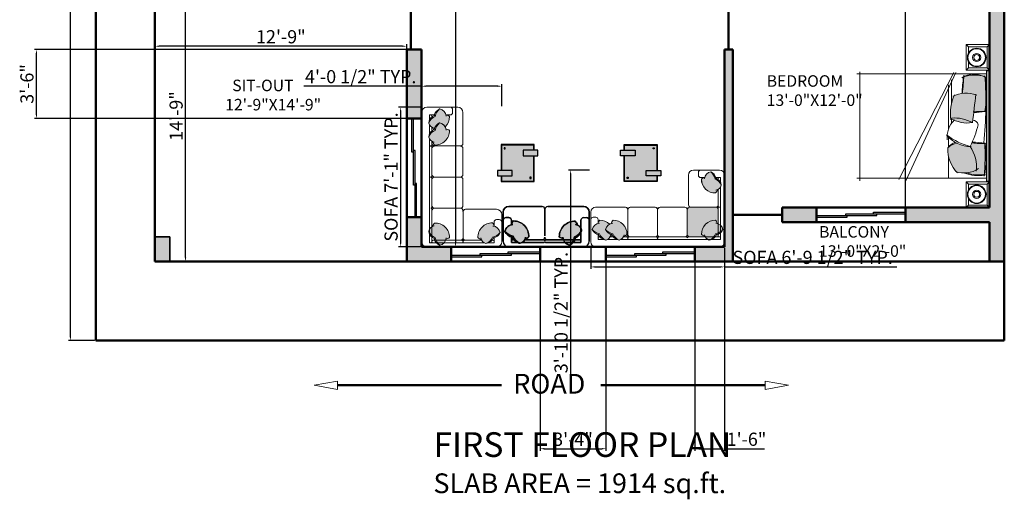
# Model space of a CAD drawing. Units: inches. Extents: x 1913 to 5309, y 1003 to 1733.
# Tile 22 of 23: x 4622 to 5221, y 1003 to 1294. Entities that reach past the tile are written whole.
import ezdxf

# ---------------------------------------------------------------- set-up
doc = ezdxf.new("R2010")
doc.units = ezdxf.units.IN
for name, color, linetype, lineweight in [('0.10', 252, 'Continuous', 9), ('0.15', 34, 'Continuous', 15), ('A-ANNO-DIMS', 2, 'Continuous', 18), ('A-ANNO-SYMB', 1, 'Continuous', 18), ('A-ANNO-TEXT', 7, 'Continuous', 18), ('A-AREA-IDEN', 3, 'Continuous', 18), ('A-COLS', 5, 'Continuous', 35), ('A-COLS-PATT', 5, 'Continuous', 13), ('A-DOOR', 4, 'Continuous', 25), ('A-FLOR-PATT', 252, 'Continuous', 13), ('A-FURN', 8, 'Continuous', 18), ('A-FURN-PATT', 8, 'Continuous', 13), ('A-GLAZ', 5, 'Continuous', 25), ('A-WALL', 7, 'Continuous', 50)]:
    doc.layers.add(name, color=color, linetype=linetype, lineweight=lineweight)
doc.layers.add('MOBIL', color=7, linetype='Continuous')
doc.styles.get("Standard").update_dxf_attribs({"font": 'arial.ttf'})
doc.dimstyles.new('ISO-25', dxfattribs={"dimtxt": 8, "dimasz": 2.5, "dimexe": 1.25, "dimexo": 0.625, "dimtad": 1, "dimdec": 1, "dimlunit": 3, "dimtxsty": 'Standard', "dimcen": 2.5, "dimclrd": 256, "dimclrt": 1, "dimadec": 0, "dimazin": 0, "dimtfac": 1, "dimtdec": 1, "dimtmove": 0, "dimatfit": 3, "dimfxl": 1, "dimarcsym": 0})

# ---------------------------------------------------------------- blocks, each defined once
blk = doc.blocks.new('Mesa de centro Cantria feeling')
at = {"layer": 'MOBIL', "ltscale": 0.2}
h = blk.add_hatch(color=256, dxfattribs=at)
h.set_gradient(color1=(74, 55, 38), color2=(104, 77, 54), one_color=1, tint=0.31, name='CYLINDER')
h.paths.add_polyline_path([(-0.85, -0.3), (-0.7, -0.3), (-0.7, 0.1), (-0.85, 0.1)])
h = blk.add_hatch(color=256, dxfattribs=at)
h.set_gradient(color1=(221, 221, 223), one_color=1, tint=1)
h.paths.add_polyline_path([(-0.15, -0.6), (-0.15, -0.89), (-0.01, -0.89), (-0.01, -0.01), (-0.7, -0.01), (-0.7, -0.3), (-0.85, -0.3), (-0.85, -0.01), (-0.99, -0.01), (-0.99, -0.89), (-0.3, -0.89), (-0.3, -0.6)])
h.paths.add_polyline_path([(-0.112, -0.112), (-0.112, -0.082), (-0.082, -0.082), (-0.082, -0.112)], flags=16)
h.paths.add_polyline_path([(-0.888, -0.788), (-0.888, -0.818), (-0.918, -0.818), (-0.918, -0.788)], flags=16)
h = blk.add_hatch(color=256, dxfattribs=at)
h.set_gradient(color1=(74, 55, 38), color2=(104, 77, 54), one_color=1, tint=0.31, name='CYLINDER')
h.paths.add_polyline_path([(-0.15, -0.6), (-0.3, -0.6), (-0.3, -1), (-0.15, -1)])
for points in [[(-0.85, 0), (-1, 0), (-1, -0.9), (-0.3, -0.9)], [(-0.15, -0.9), (0, -0.9), (0, 0), (-0.7, 0)], [(-0.85, -0.01), (-0.99, -0.01), (-0.99, -0.89), (-0.3, -0.89)], [(-0.15, -0.89), (-0.01, -0.89), (-0.01, -0.01), (-0.7, -0.01)]]:
    blk.add_lwpolyline(points, dxfattribs=at)
for points in [[(-0.85, -0.3), (-0.7, -0.3), (-0.7, 0.1), (-0.85, 0.1)], [(-0.082, -0.082), (-0.112, -0.082), (-0.112, -0.112), (-0.082, -0.112)], [(-0.918, -0.818), (-0.888, -0.818), (-0.888, -0.788), (-0.918, -0.788)], [(-0.15, -0.6), (-0.3, -0.6), (-0.3, -1), (-0.15, -1)]]:
    blk.add_lwpolyline(points, close=True, dxfattribs=at)
blk = doc.blocks.new('camita')
at = {"layer": '0.10'}
for p, q in [((-0.85, -0.045), (0.85, -0.045)), ((-0.805, -0.045), (-0.805, -2.048)), ((0.805, -0.045), (0.805, -2.048)), ((-0.827, -0.521), (0.846, -1.293)), ((-0.827, -0.548), (0.824, -1.399)), ((-0.716, -0.585), (-0.355, -0.585)), ((-0.114, -0.585), (-0.049, -0.585)), ((-0.638, -0.63), (0.043, -0.63)), ((0.175, -0.63), (0.318, -0.63)), ((0.474, -0.63), (0.805, -0.63)), ((-0.835, -2), (0.846, -2))]:
    blk.add_line(p, q, dxfattribs=at)
blk.add_lwpolyline([(-0.85, -0.041), (0.85, -0.041), (0.85, 0), (-0.85, 0)], close=True, dxfattribs=at)
for centre, radius, start, end in [((-0.457, -0.236), 0.344, 147.51, 213.8336), ((-0.2, -0.227), 0.586, 163.9263, 197.1409), ((-0.364, -5.846), 5.791, 83.8073, 94.1211), ((-0.51, -1.723), 1.678, 80.1255, 98.6619), ((2.353, -0.053), 2.58, 180.1063, 184.3854), ((-1.544, -0.245), 1.333, 359.9394, 7.5533), ((1.581, -0.289), 1.335, 170.3802, 178.9914), ((-1.44, -0.061), 1.712, 352.9291, 0.3959), ((0.452, -3.067), 3, 83.9026, 93.6759), ((0.486, -1.629), 1.578, 80.1602, 98.06), ((0.029, -0.138), 0.726, 342.5841, 6.0048), ((0.133, -0.17), 0.631, 339.923, 8.7433), ((-0.054, -0.363), 0.454, 159.3026, 206.5026), ((-1.33, -9.675), 9.499, 82.2708, 84.9399), ((0.458, -0.545), 0.584, 151.0456, 184.1497), ((-0.534, -0.339), 0.487, 327.2644, 9.0473), ((-0.007, -0.258), 0.0828, 100.018, 179.736), ((-0.293, -1.438), 1.29, 61.9749, 77.8435), ((-0.199, -0.274), 0.516, 310.7395, 359.0576), ((-0.567, -0.087), 0.906, 321.6953, 346.4626), ((0.627, -0.752), 0.551, 82.9691, 124.6739), ((0.32, -0.394), 0.404, 341.4524, 33.4512), ((-1.867, -14.986), 14.632, 84.6597, 85.7516), ((-0.46, 1.486), 1.909, 260.953, 268.6517), ((-0.2, 0.064), 0.667, 244.7809, 279.0606), ((0.179, -0.272), 0.383, 224.5284, 275.2229), ((0.438, -0.483), 0.19, 193.6849, 236.7035), ((0.571, -0.432), 0.315, 192.9388, 221.9636), ((0.361, -0.133), 0.51, 267.2589, 315.2997)]:
    blk.add_arc(centre, radius, start, end, dxfattribs=at)
blk = doc.blocks.new('VELADOR')
at = {"layer": '0.15'}
for p, q in [((-0.248, 0), (-0.203, -0.045)), ((0.248, 0), (0.202, -0.045)), ((-0.203, -0.405), (-0.248, -0.45)), ((0.248, -0.45), (0.202, -0.405))]:
    blk.add_line(p, q, dxfattribs=at)
blk.add_lwpolyline([(-0.248, 0), (-0.248, -0.45), (0.248, -0.45), (0.248, 0)], close=True, dxfattribs=at)
blk.add_lwpolyline([(0.092, -0.405), (0.202, -0.405), (0.202, -0.045), (-0.203, -0.045), (-0.203, -0.405), (-0.082, -0.405)], dxfattribs=at)
for radius in [0.18, 0.169, 0.0788, 0.0563]:
    blk.add_circle((0.005, -0.247), radius, dxfattribs=at)
blk = doc.blocks.new('d2 s')
at = {"transparency": 33554687}
h = blk.add_hatch(color=256, dxfattribs=at)
h.dxf.hatch_style = 1
h.paths.add_polyline_path([(3953.01, 1202.6, 0.213835), (3948.73, 1198.21, 0.233217), (3951.28, 1195.23, 0.122039), (3952.62, 1192.95, 0.425972), (3962.37, 1202.51, 0.156703), (3960.25, 1203.55), (3960.12, 1203.55, 0.310469), (3955.94, 1207.57, 0.147724)])
h = blk.add_hatch(color=256, dxfattribs=at)
h.dxf.hatch_style = 1
h.paths.add_polyline_path([(3953.9, 1162.75, -0.084911), (3952.59, 1164.92, -0.046133), (3950.85, 1165.51), (3950.85, 1171.8, -0.039409), (3951.63, 1172.02, -0.165523), (3952.68, 1174.28, -0.42585), (3962.24, 1164.53, -0.121928), (3959.96, 1163.19, -0.027403), (3959.75, 1162.75)])
h.paths.add_polyline_path([(3949.17, 1166.48), (3949.17, 1170.75, -0.097704), (3950.85, 1171.8), (3950.85, 1165.51, -0.04873)])
h.paths.add_polyline_path([(3947.62, 1167.84, -0.16488), (3949.17, 1170.75), (3949.17, 1166.48, -0.051917)])
h.paths.add_polyline_path([(3956, 1161.07, -0.090388), (3953.9, 1162.75), (3959.75, 1162.75, -0.136035), (3958.07, 1161.07)])
blk.add_line((3946.53, 1205.25), (3946.53, 1159.36), dxfattribs=at)
for p, q in [((3949.84, 1161.07), (3950.18, 1161.07)), ((3964.47, 1159.37), (3964.46, 1157.65))]:
    blk.add_line(p, q)
for points in [[(3955.94, 1207.57, 0.147724), (3953.01, 1202.6, 0.213355), (3948.73, 1198.22, -0.213355), (3953.01, 1202.6, -0.147724), (3955.94, 1207.57, 0.249545), (3952.4, 1203.17, -0.249545), (3955.93, 1207.59, -0.356779), (3960.22, 1202.7, 0.356779), (3955.94, 1207.57)], [(3948.72, 1198.23, 0.306333), (3952.42, 1194.91, -0.306333), (3948.72, 1198.23, -0.306674), (3952.79, 1203.29, 0.306674), (3948.72, 1198.23)], [(3952.62, 1192.95, 0.425972), (3962.37, 1202.51, 0.165552), (3960.12, 1203.57, -0.165552), (3962.37, 1202.51, -0.425972), (3952.63, 1192.95, -0.121514), (3951.29, 1195.22, 0.121514), (3952.62, 1192.95)], [(3947.62, 1167.84, 0.147724), (3952.59, 1164.92, 0.213355), (3956.97, 1160.64, -0.213355), (3952.59, 1164.92, -0.147724), (3947.62, 1167.84, 0.249545), (3952.02, 1164.3, -0.249545), (3947.61, 1167.84, -0.356779), (3952.49, 1172.13, 0.356779), (3947.62, 1167.84)], [(3962.24, 1164.53, 0.425972), (3952.68, 1174.28, 0.165552), (3951.63, 1172.02, -0.165552), (3952.68, 1174.28, -0.425972), (3962.24, 1164.53, -0.121514), (3959.97, 1163.19, 0.121514), (3962.24, 1164.53)], [(3956.96, 1160.63, 0.306333), (3960.28, 1164.33, -0.306333), (3956.96, 1160.63, -0.306674), (3951.9, 1164.7, 0.306674), (3956.96, 1160.63)]]:
    blk.add_lwpolyline(points, format="xyb", dxfattribs=at)
for points in [[(3949.93, 1208.66), (3967.86, 1208.66)], [(3964.46, 1205.25), (3964.46, 1206.96)], [(3949.17, 1203.55), (3952.49, 1203.55), (3949.17, 1203.55), (3949.17, 1199.96)], [(3950.85, 1202.87), (3950.85, 1202.25)], [(3960.13, 1203.55), (3962.77, 1203.55)], [(3971.27, 1205.25), (3971.27, 1184.84)], [(3949.17, 1197.14), (3949.17, 1183.83)], [(3950.85, 1195.43), (3950.85, 1183.83)], [(3949.17, 1164.09), (3949.17, 1182.51)], [(3950.99, 1183.17), (3950.65, 1183.17)], [(3950.85, 1161.74), (3950.85, 1182.51)], [(3969.63, 1183.17), (3953.36, 1183.17)], [(3971.25, 1181.39), (3971.25, 1159.35)], [(3949.17, 1161.07), (3949.17, 1164.4), (3949.17, 1161.07), (3952.75, 1161.07)], [(3952.75, 1161.06), (3962.77, 1161.06)], [(3949.93, 1155.95), (3967.86, 1155.95)]]:
    blk.add_lwpolyline(points, close=True, dxfattribs=at)
for points in [[(3962.76, 1208.66, -0.414214), (3964.46, 1206.97, 0.414214)], [(3967.85, 1208.66, -0.414212), (3971.25, 1205.26, 0.414212)], [(3950.18, 1203.55, -0.414214), (3950.85, 1202.88, 0.414214)], [(3964.46, 1205.26, -0.414214), (3962.76, 1203.57, 0.414214)], [(3964.47, 1159.37, 0.414214), (3962.77, 1161.06, -0.414214)], [(3967.85, 1155.95, 0.414212), (3971.25, 1159.35, -0.414212)], [(3962.76, 1155.95, 0.414214), (3964.46, 1157.65, -0.414214)]]:
    blk.add_lwpolyline(points, format="xyb", close=True, dxfattribs=at)
for centre, radius, start, end in [((3949.93, 1205.26), 3.4, 90.00019, 179.99981), ((3949.93, 1205.26), 3.4, 90.08458, 180.08419), ((3949.85, 1183.85), 0.681, 179.15747, 269.15748), ((3949.85, 1182.49), 0.681, 90.84252, 180.84253), ((3950.18, 1183.84), 0.671, 270, 0), ((3950.18, 1183.84), 0.671, 270, 0), ((3950.18, 1182.5), 0.671, 360, 90), ((3950.18, 1182.5), 0.671, 360, 90), ((3952.51, 1184.83), 1.66, 179.48888, 271.23403), ((3952.51, 1181.52), 1.66, 88.76597, 180.51112), ((3969.59, 1184.83), 1.66, 268.766, 0.51111), ((3969.39, 1181.32), 1.86, 2.05774, 84.98178), ((3969.39, 1181.32), 1.86, 2.05774, 84.98178), ((3969.59, 1184.83), 1.66, 268.7816, 0.51111), ((3949.93, 1159.36), 3.4, 180.00019, 269.99981), ((3949.93, 1159.37), 3.4, 180.08458, 270.08419), ((3949.84, 1161.74), 0.671, 180, 270), ((3950.18, 1161.74), 0.671, 270, 0)]:
    blk.add_arc(centre, radius, start, end, dxfattribs=at)
blk = doc.blocks.new('SOFA 1')
at = {"transparency": 33554687}
h = blk.add_hatch(color=256, dxfattribs=at)
h.dxf.hatch_style = 1
h.paths.add_polyline_path([(3723.52, 1308.63, 0.147724), (3717.76, 1305.24, 0.310469), (3722.42, 1300.4), (3722.42, 1300.25, 0.156703), (3723.62, 1297.8, 0.425821), (3734.69, 1309.08, 0.121928), (3732.05, 1310.63, 0.233216), (3728.6, 1313.59, 0.213835)])
h = blk.add_hatch(color=256, dxfattribs=at)
h.dxf.hatch_style = 1
h.paths.add_polyline_path([(3769.65, 1307.6, 0.084911), (3767.15, 1309.12, 0.046133), (3766.46, 1311.13), (3759.18, 1311.13, 0.039409), (3758.92, 1310.24, 0.165523), (3756.31, 1309.02, 0.42585), (3767.59, 1297.95, 0.121928), (3769.15, 1300.58, 0.027403), (3769.65, 1300.83)])
h.paths.add_polyline_path([(3765.34, 1313.08), (3760.4, 1313.08, 0.097704), (3759.18, 1311.13), (3766.46, 1311.13, 0.04873)])
h.paths.add_polyline_path([(3763.76, 1314.88, 0.16488), (3760.4, 1313.08), (3765.34, 1313.08, 0.051917)])
h.paths.add_polyline_path([(3771.6, 1305.17, 0.090388), (3769.65, 1307.6), (3769.65, 1300.83, 0.136035), (3771.6, 1302.77)])
h = blk.add_hatch(color=256, dxfattribs=at)
h.dxf.hatch_style = 1
h.paths.add_polyline_path([(3769.16, 1235.96, 0.122267), (3767.6, 1238.61, 0.425972), (3756.32, 1227.54, 0.165563), (3758.93, 1226.32, 0.309481), (3763.76, 1221.69, 0.002677), (3763.83, 1221.72, 0.146094), (3767.16, 1227.43, 0.212433), (3772.1, 1232.48, 0.235342)])
h = blk.add_hatch(color=256, dxfattribs=at)
h.dxf.hatch_style = 1
h.paths.add_polyline_path([(3769.16, 1225.36, 0.122267), (3767.6, 1228.01, 0.425972), (3756.32, 1216.94, 0.165563), (3758.93, 1215.72, 0.309481), (3763.76, 1211.09, 0.002677), (3763.83, 1211.12, 0.146094), (3767.16, 1216.83, 0.212433), (3772.1, 1221.88, 0.235342)])
for p, q in [((3720.45, 1316.13), (3773.58, 1316.13)), ((3777.51, 1312.19), (3777.51, 1213.72))]:
    blk.add_line(p, q, dxfattribs=at)
for points in [[(3716.51, 1312.2), (3716.51, 1291.44)], [(3722.42, 1313.08), (3722.42, 1309.23), (3722.42, 1313.08), (3726.57, 1313.08)], [(3723.21, 1311.13), (3723.93, 1311.13)], [(3729.85, 1313.08), (3745.25, 1313.08)], [(3731.82, 1311.13), (3745.25, 1311.13)], [(3746.01, 1312.3), (3746.01, 1288.55)], [(3746.01, 1310.97), (3746.01, 1311.36)], [(3768.11, 1313.08), (3746.78, 1313.08)], [(3768.87, 1311.13), (3746.78, 1311.13)], [(3771.6, 1313.08), (3767.75, 1313.08), (3771.6, 1313.08), (3771.6, 1308.93)], [(3769.66, 1287.39), (3769.65, 1312.3)], [(3771.6, 1313.08), (3771.61, 1233.74)], [(3746.01, 1288.54), (3746.01, 1308.23)], [(3769.65, 1309.43), (3769.65, 1308.71)], [(3722.42, 1300.39), (3722.42, 1297.33)], [(3720.45, 1295.38), (3718.48, 1295.38)], [(3720.45, 1287.5), (3744.09, 1287.5)], [(3746.02, 1284.63), (3746.02, 1264.94)], [(3747.99, 1286.6), (3767.69, 1286.6)], [(3769.66, 1263.75), (3769.66, 1285.81)], [(3769.66, 1277.18), (3769.66, 1263.75)], [(3746.02, 1260.99), (3746.02, 1241.3)], [(3747.99, 1262.97), (3767.69, 1262.97)], [(3769.66, 1240.12), (3769.66, 1262.18)], [(3770.43, 1262.97), (3770.82, 1262.97)], [(3746.02, 1237.36), (3746.02, 1213.74)], [(3747.99, 1239.33), (3767.69, 1239.33)], [(3769.66, 1235.71), (3769.66, 1238.54)], [(3770.43, 1239.33), (3770.82, 1239.33)], [(3771.61, 1223.14), (3771.61, 1230.47)], [(3769.66, 1225.11), (3769.66, 1227.82)], [(3753.91, 1211.77), (3753.91, 1213.74)], [(3755.86, 1215.72), (3758.92, 1215.72)], [(3767.76, 1215.72), (3771.61, 1215.72), (3771.61, 1219.84), (3771.61, 1215.72)], [(3769.66, 1216.5), (3769.66, 1217.22)], [(3749.97, 1209.8), (3773.58, 1209.8)]]:
    blk.add_lwpolyline(points, close=True, dxfattribs=at)
for points in [[(3717.76, 1305.24, -0.147724), (3723.52, 1308.63, -0.213355), (3728.59, 1313.59, 0.213355), (3723.52, 1308.63, 0.147724), (3717.76, 1305.24, -0.249545), (3722.86, 1309.34, 0.249545), (3717.75, 1305.25, 0.356779), (3723.4, 1300.28, -0.356779), (3717.76, 1305.24)], [(3728.58, 1313.6, -0.306333), (3732.42, 1309.31, 0.306333), (3728.58, 1313.6, 0.306674), (3722.72, 1308.89, -0.306674), (3728.58, 1313.6)], [(3763.76, 1314.88, -0.147724), (3767.15, 1309.12, -0.213355), (3772.1, 1304.05, 0.213355), (3767.15, 1309.12, 0.147724), (3763.76, 1314.88, -0.249545), (3767.86, 1309.77, 0.249545), (3763.77, 1314.89, 0.356779), (3758.8, 1309.23, -0.356779), (3763.76, 1314.88)], [(3734.69, 1309.08, -0.425972), (3723.62, 1297.8, -0.165552), (3722.4, 1300.4, 0.165552), (3723.62, 1297.79, 0.425972), (3734.69, 1309.07, 0.121514), (3732.07, 1310.63, -0.121514), (3734.69, 1309.08)], [(3767.6, 1297.95, -0.425972), (3756.31, 1309.01, -0.165552), (3758.92, 1310.24, 0.165552), (3756.31, 1309.02, 0.425972), (3767.59, 1297.95, 0.121514), (3769.14, 1300.57, -0.121514), (3767.6, 1297.95)], [(3772.11, 1304.06, -0.306333), (3767.83, 1300.22, 0.306333), (3772.11, 1304.06, 0.306674), (3767.4, 1309.91, -0.306674), (3772.11, 1304.06)], [(3770.44, 1286.63, -0.414214), (3769.66, 1287.4, 0.414214), (3770.44, 1286.63, 0.414214), (3769.66, 1285.83, -0.414214), (3770.44, 1286.63)], [(3748.01, 1262.99, -0.414214), (3746.05, 1264.95, 0.414214), (3748.01, 1262.97, 0.414213), (3746.05, 1261.01, -0.414213), (3748.01, 1262.99)], [(3770.44, 1262.99, -0.414214), (3769.66, 1263.77, 0.414214), (3770.44, 1262.99, 0.414214), (3769.66, 1262.19, -0.414214), (3770.44, 1262.99)], [(3770.83, 1262.97, -0.414214), (3771.61, 1262.19, 0.414214), (3770.83, 1262.99, 0.414214), (3771.61, 1263.77, -0.414214), (3770.83, 1262.97)], [(3748.01, 1239.35, -0.414214), (3746.05, 1241.31, 0.414214), (3748.01, 1239.33, 0.414213), (3746.05, 1237.37, -0.414213), (3748.01, 1239.35)], [(3756.32, 1227.54, -0.425972), (3767.6, 1238.61, -0.121514), (3769.16, 1235.98, 0.121514), (3767.6, 1238.61, 0.425972), (3756.32, 1227.54, 0.165552), (3758.93, 1226.32, -0.165552), (3756.32, 1227.54)], [(3772.1, 1232.5, -0.306674), (3767.41, 1226.64, 0.306674), (3772.1, 1232.5, 0.306333), (3767.84, 1236.34, -0.306333), (3772.1, 1232.5)], [(3767.7, 1239.33, -0.414214), (3769.66, 1237.37, 0.414214), (3767.7, 1239.35, 0.414214), (3769.66, 1241.31, -0.414214), (3767.7, 1239.33)], [(3770.44, 1239.35, -0.414214), (3769.66, 1240.13, 0.414214), (3770.44, 1239.33, 0.414214), (3769.66, 1238.55, -0.414214), (3770.44, 1239.35)], [(3770.83, 1239.33, -0.414214), (3771.61, 1238.55, 0.414214), (3770.83, 1239.35, 0.414214), (3771.61, 1240.13, -0.414214), (3770.83, 1239.33)], [(3763.78, 1221.67, 0.249545), (3767.87, 1226.78, -0.249545), (3763.76, 1221.69, -0.356779), (3758.81, 1227.32, 0.356779), (3763.77, 1221.68, 0.147724), (3767.16, 1227.43, 0.213355), (3772.11, 1232.51, -0.213355), (3767.16, 1227.43, -0.147724), (3763.78, 1221.67)], [(3756.32, 1216.94, -0.200233), (3759.49, 1224.76, 0.200233), (3756.32, 1216.94, 0.165552), (3758.93, 1215.72, -0.165552), (3756.32, 1216.94)], [(3772.1, 1221.9, -0.306674), (3767.41, 1216.04, 0.306674), (3772.1, 1221.9, -0.213355), (3767.16, 1216.83, -0.147724), (3763.77, 1211.08, 0.147724), (3767.15, 1216.83, 0.213355), (3772.1, 1221.9)], [(3763.76, 1211.09, -0.356779), (3758.81, 1216.72, 0.356779), (3763.76, 1211.09, 0.249545), (3767.87, 1216.18, -0.249545), (3763.76, 1211.09)]]:
    blk.add_lwpolyline(points, format="xyb", dxfattribs=at)
for points in [[(3722.42, 1311.91, 0.414214), (3723.2, 1311.13, -0.414214)], [(3770.43, 1313.08, 0.414214), (3769.65, 1312.3, -0.414214)], [(3771.6, 1312.3, 0.414214), (3770.82, 1313.08, -0.414214)], [(3716.51, 1297.34, 0.414214), (3718.47, 1295.38, -0.414214)], [(3720.44, 1295.38, 0.414214), (3722.4, 1297.34, -0.414214)], [(3716.51, 1291.45, 0.414212), (3720.44, 1287.52, -0.414212)], [(3746.03, 1288.56, 0.414214), (3747.99, 1286.6, 0.414213), (3746.03, 1284.64, -0.414213), (3747.99, 1286.6, -0.414214)], [(3769.66, 1284.64, 0.414214), (3767.7, 1286.6, 0.414214), (3769.66, 1288.56, -0.414214), (3767.7, 1286.6, -0.414214)], [(3769.66, 1261.01, 0.414214), (3767.7, 1262.97, 0.414214), (3769.66, 1264.93, -0.414214), (3767.7, 1262.97, -0.414214)], [(3772.13, 1221.9, 0.306333), (3767.84, 1225.74, -0.306333)], [(3769.16, 1225.36, 0.071861), (3768.39, 1227.01, -0.071861)], [(3746.05, 1213.76, 0.414212), (3749.98, 1209.82, -0.414212)], [(3755.87, 1215.72, 0.414214), (3753.91, 1213.76, -0.414214)], [(3769.66, 1216.52, 0.414214), (3770.44, 1215.74, -0.414214)], [(3770.83, 1215.74, 0.414214), (3771.61, 1216.52, -0.414214)], [(3755.87, 1209.8, -0.414214), (3753.91, 1211.76, 0.414214)]]:
    blk.add_lwpolyline(points, format="xyb", close=True, dxfattribs=at)
for centre, radius, start, end in [((3720.44, 1312.2), 3.93, 90.00019, 179.99981), ((3720.44, 1312.19), 3.94, 89.91581, 179.91542), ((3744.09, 1309.21), 1.92, 358.76597, 90.51112), ((3745.22, 1312.29), 0.789, 0.84252, 90.84253), ((3745.24, 1311.91), 0.777, 270, 0), ((3745.24, 1311.91), 0.777, 270, 0), ((3746.8, 1312.29), 0.789, 89.15747, 179.15748), ((3746.79, 1311.91), 0.777, 180, 270), ((3746.79, 1311.91), 0.777, 180, 270), ((3747.93, 1309.21), 1.92, 89.48888, 181.23403), ((3768.87, 1312.3), 0.777, 360, 90), ((3768.87, 1311.91), 0.777, 270, 0), ((3773.58, 1312.2), 3.93, 0.00019, 89.99981), ((3773.57, 1312.19), 3.94, 359.91581, 89.91542), ((3744.08, 1289.48), 1.96, 270, 360), ((3744.08, 1289.48), 1.96, 270, 360), ((3773.58, 1213.73), 3.93, 270.00019, 359.99981), ((3773.59, 1213.73), 3.93, 269.91556, 359.91517)]:
    blk.add_arc(centre, radius, start, end, dxfattribs=at)
blk = doc.blocks.new('*D29')
at = {"layer": 'A-ANNO-DIMS', "color": 0, "lineweight": -2, "transparency": 16777216}
for p, q in [((4668.01, 1686.96), (4652.03, 1686.96)), ((4653.28, 1101.46), (4653.28, 1684.46)), ((4668.01, 1098.96), (4652.03, 1098.96))]:
    blk.add_line(p, q, dxfattribs=at)
at = {"layer": 'A-ANNO-DIMS', "color": 0, "transparency": 16777216}
for points in [[(4652.86, 1684.46), (4653.69, 1684.46), (4653.28, 1686.96)], [(4652.86, 1101.46), (4653.69, 1101.46), (4653.28, 1098.96)]]:
    blk.add_solid(points, dxfattribs=at)
at = {"layer": 'Defpoints', "color": 0, "transparency": 16777216}
for p in [(4653.28, 1686.96), (4668.63, 1686.96), (4668.63, 1098.96)]:
    blk.add_point(p, dxfattribs=at)
at = {"layer": 'A-ANNO-DIMS', "color": 0, "transparency": 16777216, "insert": (4648.57, 1392.96), "char_height": 8, "attachment_point": 5, "rotation": 90}
blk.add_mtext("49'", dxfattribs=at)
blk = doc.blocks.new('*D33')
at = {"layer": 'A-ANNO-DIMS', "color": 0, "lineweight": -2, "transparency": 16777216}
for p, q in [((4722.69, 1323.96), (4724.5, 1323.96)), ((4723.25, 1149.46), (4723.25, 1321.46)), ((4722.69, 1146.96), (4724.5, 1146.96))]:
    blk.add_line(p, q, dxfattribs=at)
at = {"layer": 'A-ANNO-DIMS', "color": 0, "transparency": 16777216}
for points in [[(4722.83, 1321.46), (4723.66, 1321.46), (4723.25, 1323.96)], [(4722.83, 1149.46), (4723.66, 1149.46), (4723.25, 1146.96)]]:
    blk.add_solid(points, dxfattribs=at)
at = {"layer": 'Defpoints', "color": 0, "transparency": 16777216}
for p in [(4722.06, 1323.96), (4723.25, 1323.96), (4722.06, 1146.96)]:
    blk.add_point(p, dxfattribs=at)
at = {"layer": 'A-ANNO-DIMS', "color": 0, "transparency": 16777216, "insert": (4718.54, 1235.46), "char_height": 8, "attachment_point": 5, "rotation": 90}
blk.add_mtext('14\'-9"', dxfattribs=at)
blk = doc.blocks.new('*D34')
at = {"layer": 'A-ANNO-DIMS', "color": 0, "lineweight": -2, "transparency": 16777216}
for p, q in [((4704.63, 1276.59), (4704.63, 1279.13)), ((4855.13, 1277.88), (4707.13, 1277.88)), ((4857.63, 1276.59), (4857.63, 1279.13))]:
    blk.add_line(p, q, dxfattribs=at)
at = {"layer": 'A-ANNO-DIMS', "color": 0, "transparency": 16777216}
for points in [[(4707.13, 1278.3), (4707.13, 1277.47), (4704.63, 1277.88)], [(4855.13, 1278.3), (4855.13, 1277.47), (4857.63, 1277.88)]]:
    blk.add_solid(points, dxfattribs=at)
at = {"layer": 'Defpoints', "color": 0, "transparency": 16777216}
for p in [(4704.63, 1277.88), (4704.63, 1275.96), (4857.63, 1275.96)]:
    blk.add_point(p, dxfattribs=at)
at = {"layer": 'A-ANNO-DIMS', "color": 0, "transparency": 16777216, "insert": (4781.13, 1282.59), "char_height": 8, "attachment_point": 5}
blk.add_mtext('12\'-9"', dxfattribs=at)
blk = doc.blocks.new('*D39')
at = {"layer": 'A-ANNO-DIMS', "color": 0, "lineweight": -2, "transparency": 16777216}
for p, q in [((4881.23, 1599.96), (4888.52, 1599.96)), ((4887.27, 1597.46), (4887.27, 1158.43)), ((4881.23, 1155.93), (4888.52, 1155.93))]:
    blk.add_line(p, q, dxfattribs=at)
at = {"layer": 'A-ANNO-DIMS', "color": 0, "transparency": 16777216}
for points in [[(4886.85, 1597.46), (4887.69, 1597.46), (4887.27, 1599.96)], [(4886.85, 1158.43), (4887.69, 1158.43), (4887.27, 1155.93)]]:
    blk.add_solid(points, dxfattribs=at)
at = {"layer": 'Defpoints', "color": 0, "transparency": 16777216}
for p in [(4880.6, 1599.96), (4880.6, 1155.93), (4887.27, 1155.93)]:
    blk.add_point(p, dxfattribs=at)
at = {"layer": 'A-ANNO-DIMS', "color": 0, "transparency": 16777216, "insert": (4882.56, 1377.95), "char_height": 8, "attachment_point": 5, "rotation": 90}
blk.add_mtext("37'", dxfattribs=at)
blk = doc.blocks.new('WIN-54')
for p, q in [((0, 54), (0, 35)), ((1, 54), (1, 17)), ((1, 36), (2, 36)), ((2, 36), (2, 0)), ((0, 35), (1, 35)), ((2, 19), (3, 19)), ((3, 19), (3, 0)), ((1, 17), (2, 17))]:
    blk.add_line(p, q)
blk = doc.blocks.new('WIN-60')
for p, q in [((0, 60), (0, 39.5)), ((1, 60), (1, 19.5)), ((0, 39.5), (1, 39.5)), ((1, 40.5), (2, 40.5)), ((2, 40.5), (2, 0)), ((1, 19.5), (2, 19.5)), ((2, 20.5), (3, 20.5)), ((3, 20.5), (3, 0))]:
    blk.add_line(p, q)
blk = doc.blocks.new('*D65')
at = {"layer": 'A-ANNO-DIMS', "color": 0, "lineweight": -2, "transparency": 16777216}
for p, q in [((4969.35, 1155.34), (4969.35, 1142.52)), ((5050.64, 1155.34), (5050.64, 1142.52))]:
    blk.add_line(p, q, dxfattribs=at)
at = {"layer": 'A-ANNO-DIMS', "lineweight": -2, "transparency": 16777216}
for p, q in [((4971.85, 1143.77), (5048.14, 1143.77)), ((5050.64, 1143.77), (5155.29, 1143.77))]:
    blk.add_line(p, q, dxfattribs=at)
at = {"layer": 'A-ANNO-DIMS', "transparency": 16777216}
for points in [[(4971.85, 1144.18), (4971.85, 1143.35), (4969.35, 1143.77)], [(5048.14, 1144.18), (5048.14, 1143.35), (5050.64, 1143.77)]]:
    blk.add_solid(points, dxfattribs=at)
at = {"layer": 'Defpoints', "color": 0, "transparency": 16777216}
for p in [(4969.35, 1155.96), (5050.64, 1155.96), (5050.64, 1143.77)]:
    blk.add_point(p, dxfattribs=at)
at = {"layer": 'A-ANNO-DIMS', "color": 1, "transparency": 16777216, "insert": (5104.21, 1148.53), "char_height": 8, "attachment_point": 5}
blk.add_mtext('SOFA 6\'-9 1/2" TYP.', dxfattribs=at)
blk = doc.blocks.new('*D66')
at = {"layer": 'A-ANNO-DIMS', "color": 0, "lineweight": -2, "transparency": 16777216}
for p, q in [((4968.73, 1202.59), (4955.91, 1202.59)), ((4968.73, 1155.96), (4955.91, 1155.96))]:
    blk.add_line(p, q, dxfattribs=at)
at = {"layer": 'A-ANNO-DIMS', "lineweight": -2, "transparency": 16777216}
for p, q in [((4957.16, 1200.09), (4957.16, 1158.46)), ((4957.16, 1155.96), (4957.16, 1078.6))]:
    blk.add_line(p, q, dxfattribs=at)
at = {"layer": 'A-ANNO-DIMS', "transparency": 16777216}
for points in [[(4956.74, 1200.09), (4957.58, 1200.09), (4957.16, 1202.59)], [(4956.74, 1158.46), (4957.58, 1158.46), (4957.16, 1155.96)]]:
    blk.add_solid(points, dxfattribs=at)
at = {"layer": 'Defpoints', "color": 0, "transparency": 16777216}
for p in [(4969.35, 1202.59), (4957.16, 1155.96), (4969.35, 1155.96)]:
    blk.add_point(p, dxfattribs=at)
at = {"layer": 'A-ANNO-DIMS', "color": 1, "transparency": 16777216, "insert": (4952.4, 1116.03), "char_height": 8, "attachment_point": 5, "rotation": 90}
blk.add_mtext('3\'-10 1/2" TYP.', dxfattribs=at)
blk = doc.blocks.new('*D67')
at = {"layer": 'A-ANNO-DIMS', "color": 0, "lineweight": -2, "transparency": 16777216}
for p, q in [((4866.01, 1240.84), (4852.64, 1240.84)), ((4866.01, 1155.93), (4852.64, 1155.93))]:
    blk.add_line(p, q, dxfattribs=at)
at = {"layer": 'A-ANNO-DIMS', "lineweight": -2, "transparency": 16777216}
blk.add_line((4853.89, 1238.34), (4853.89, 1158.43), dxfattribs=at)
at = {"layer": 'A-ANNO-DIMS', "transparency": 16777216}
for points in [[(4853.48, 1238.34), (4854.31, 1238.34), (4853.89, 1240.84)], [(4853.48, 1158.43), (4854.31, 1158.43), (4853.89, 1155.93)]]:
    blk.add_solid(points, dxfattribs=at)
at = {"layer": 'Defpoints', "color": 0, "transparency": 16777216}
for p in [(4866.63, 1240.84), (4853.89, 1155.93), (4866.63, 1155.93)]:
    blk.add_point(p, dxfattribs=at)
at = {"layer": 'A-ANNO-DIMS', "color": 1, "transparency": 16777216, "insert": (4849.13, 1198.39), "char_height": 8, "attachment_point": 5, "rotation": 90}
blk.add_mtext('SOFA 7\'-1" TYP.', dxfattribs=at)
blk = doc.blocks.new('*D68')
at = {"layer": 'A-ANNO-DIMS', "lineweight": -2, "transparency": 16777216}
for p, q in [((4866.63, 1253.58), (4795.15, 1253.58)), ((4912.85, 1253.58), (4869.13, 1253.58))]:
    blk.add_line(p, q, dxfattribs=at)
at = {"layer": 'A-ANNO-DIMS', "color": 0, "lineweight": -2, "transparency": 16777216}
for p, q in [((4866.63, 1241.47), (4866.63, 1254.83)), ((4915.35, 1241.47), (4915.35, 1254.83))]:
    blk.add_line(p, q, dxfattribs=at)
at = {"layer": 'A-ANNO-DIMS', "transparency": 16777216}
for points in [[(4869.13, 1254), (4869.13, 1253.16), (4866.63, 1253.58)], [(4912.85, 1254), (4912.85, 1253.16), (4915.35, 1253.58)]]:
    blk.add_solid(points, dxfattribs=at)
at = {"layer": 'Defpoints', "color": 0, "transparency": 16777216}
for p in [(4866.63, 1253.58), (4866.63, 1240.84), (4915.35, 1240.84)]:
    blk.add_point(p, dxfattribs=at)
at = {"layer": 'A-ANNO-DIMS', "color": 1, "transparency": 16777216, "insert": (4829.64, 1258.34), "char_height": 8, "attachment_point": 5}
blk.add_mtext('4\'-0 1/2" TYP.', dxfattribs=at)
blk = doc.blocks.new('*D135')
at = {"layer": 'A-ANNO-DIMS', "color": 0, "lineweight": -2, "transparency": 16777216}
for p, q in [((5032.63, 1155.34), (5032.63, 1032.04)), ((5050.63, 1155.34), (5050.63, 1032.04))]:
    blk.add_line(p, q, dxfattribs=at)
at = {"layer": 'A-ANNO-DIMS', "lineweight": -2, "transparency": 16777216}
for p, q in [((5035.13, 1033.29), (5048.13, 1033.29)), ((5050.63, 1033.29), (5074.9, 1033.29))]:
    blk.add_line(p, q, dxfattribs=at)
at = {"layer": 'A-ANNO-DIMS', "transparency": 16777216}
for points in [[(5035.13, 1033.7), (5035.13, 1032.87), (5032.63, 1033.29)], [(5048.13, 1033.7), (5048.13, 1032.87), (5050.63, 1033.29)]]:
    blk.add_solid(points, dxfattribs=at)
at = {"layer": 'Defpoints', "color": 0, "transparency": 16777216}
for p in [(5032.63, 1155.96), (5050.63, 1155.96), (5050.63, 1033.29)]:
    blk.add_point(p, dxfattribs=at)
at = {"layer": 'A-ANNO-DIMS', "color": 1, "transparency": 16777216, "insert": (5064.02, 1038), "char_height": 8, "attachment_point": 5}
blk.add_mtext('1\'-6"', dxfattribs=at)
blk = doc.blocks.new('*D136')
at = {"layer": 'A-ANNO-DIMS', "color": 0, "lineweight": -2, "transparency": 16777216}
for p, q in [((4938.63, 1146.34), (4938.63, 1032.04)), ((4978.63, 1146.34), (4978.63, 1032.04))]:
    blk.add_line(p, q, dxfattribs=at)
at = {"layer": 'A-ANNO-DIMS', "lineweight": -2, "transparency": 16777216}
blk.add_line((4941.13, 1033.29), (4976.13, 1033.29), dxfattribs=at)
at = {"layer": 'A-ANNO-DIMS', "transparency": 16777216}
for points in [[(4941.13, 1033.7), (4941.13, 1032.87), (4938.63, 1033.29)], [(4976.13, 1033.7), (4976.13, 1032.87), (4978.63, 1033.29)]]:
    blk.add_solid(points, dxfattribs=at)
at = {"layer": 'Defpoints', "color": 0, "transparency": 16777216}
for p in [(4938.63, 1146.96), (4978.63, 1146.96), (4978.63, 1033.29)]:
    blk.add_point(p, dxfattribs=at)
at = {"layer": 'A-ANNO-DIMS', "color": 1, "transparency": 16777216, "insert": (4958.63, 1038), "char_height": 8, "attachment_point": 5}
blk.add_mtext('3\'-4"', dxfattribs=at)
blk = doc.blocks.new('*D137')
at = {"layer": 'A-ANNO-DIMS', "color": 0, "lineweight": -2, "transparency": 16777216}
for p, q in [((4866.01, 1275.96), (4631.38, 1275.96)), ((4866.01, 1233.96), (4631.38, 1233.96))]:
    blk.add_line(p, q, dxfattribs=at)
at = {"layer": 'A-ANNO-DIMS', "lineweight": -2, "transparency": 16777216}
blk.add_line((4632.63, 1236.46), (4632.63, 1273.46), dxfattribs=at)
at = {"layer": 'A-ANNO-DIMS', "transparency": 16777216}
for points in [[(4632.22, 1273.46), (4633.05, 1273.46), (4632.63, 1275.96)], [(4632.22, 1236.46), (4633.05, 1236.46), (4632.63, 1233.96)]]:
    blk.add_solid(points, dxfattribs=at)
at = {"layer": 'Defpoints', "color": 0, "transparency": 16777216}
for p in [(4632.63, 1275.96), (4866.63, 1275.96), (4866.63, 1233.96)]:
    blk.add_point(p, dxfattribs=at)
at = {"layer": 'A-ANNO-DIMS', "color": 1, "transparency": 16777216, "insert": (4627.92, 1254.96), "char_height": 8, "attachment_point": 5, "rotation": 90}
blk.add_mtext('3\'-6"', dxfattribs=at)
blk = doc.blocks.new('*D138')
at = {"layer": 'A-ANNO-DIMS', "color": 0, "lineweight": -2, "transparency": 16777216}
for p, q in [((5160.63, 1180.59), (5160.63, 1724.21)), ((5211.63, 1180.59), (5211.63, 1724.21))]:
    blk.add_line(p, q, dxfattribs=at)
at = {"layer": 'A-ANNO-DIMS', "lineweight": -2, "transparency": 16777216}
blk.add_line((5163.13, 1722.96), (5209.13, 1722.96), dxfattribs=at)
at = {"layer": 'A-ANNO-DIMS', "transparency": 16777216}
for points in [[(5163.13, 1723.38), (5163.13, 1722.55), (5160.63, 1722.96)], [(5209.13, 1723.38), (5209.13, 1722.55), (5211.63, 1722.96)]]:
    blk.add_solid(points, dxfattribs=at)
at = {"layer": 'Defpoints', "color": 0, "transparency": 16777216}
for p in [(5211.63, 1722.96), (5160.63, 1179.96), (5211.63, 1179.96)]:
    blk.add_point(p, dxfattribs=at)
at = {"layer": 'A-ANNO-DIMS', "color": 1, "transparency": 16777216, "insert": (5186.13, 1727.68), "char_height": 8, "attachment_point": 5}
blk.add_mtext('4\'-3"', dxfattribs=at)

msp = doc.modelspace()

# ---------------------------------------------------------------- hatches: boundary and pattern name
at = {"layer": 'A-COLS-PATT'}
h = msp.add_hatch(color=256, dxfattribs=at)
h.dxf.hatch_style = 1
h.paths.add_polyline_path([(4713.63, 1161.96), (4704.63, 1161.96), (4704.63, 1146.96), (4713.63, 1146.96)])
at = {"layer": 'A-FLOR-PATT'}
h = msp.add_hatch(color=256, dxfattribs=at)
h.dxf.hatch_style = 1
h.paths.add_polyline_path([(4862.63, 1686.96), (4704.63, 1686.96), (4704.63, 1625.96), (4713.63, 1625.96), (4713.63, 1677.96), (4857.63, 1677.96), (4857.63, 1554.96), (4862.63, 1554.96), (4862.63, 1599.96), (4880.6, 1599.96), (4880.6, 1608.96), (4862.63, 1608.96)])
h.paths.add_polyline_path([(5055.63, 1625.46), (5050.63, 1625.46), (5050.63, 1608.96), (4976.6, 1608.96), (4976.6, 1599.96), (5050.63, 1599.96), (5050.63, 1528.96), (5055.63, 1528.96)])
h.paths.add_polyline_path([(5220.63, 1686.96), (5050.63, 1686.96), (5050.63, 1661.46), (5055.63, 1661.46), (5055.63, 1677.96), (5211.63, 1677.96), (5211.63, 1492.96), (5050.63, 1492.96), (5050.63, 1487.96), (5179.63, 1487.96), (5179.63, 1464.96), (5184.63, 1464.96), (5184.63, 1487.96), (5220.63, 1487.96)])
h.paths.add_polyline_path([(5120.63, 1400.96), (5184.63, 1400.96), (5184.63, 1428.96), (5179.63, 1428.96), (5179.63, 1405.96), (5050.63, 1405.96), (5050.63, 1311.96), (5055.63, 1311.96), (5055.63, 1323.96), (5079.63, 1323.96), (5079.63, 1328.96), (5055.63, 1328.96), (5055.63, 1400.96), (5115.63, 1400.96), (5115.63, 1358.96), (5120.63, 1358.96)])
h.paths.add_polyline_path([(5220.63, 1405.96), (5208.63, 1405.96), (5208.63, 1400.96), (5211.63, 1400.96), (5211.63, 1328.96), (5115.63, 1328.96), (5115.63, 1323.96), (5211.63, 1323.96), (5211.63, 1299.96), (5211.63, 1179.96), (5197.5, 1179.96), (5160.63, 1179.96), (5160.63, 1170.96), (5211.63, 1170.96), (5211.63, 1146.96), (5220.63, 1146.96)])
h.paths.add_polyline_path([(5106.63, 1179.96), (5085.63, 1179.96), (5085.63, 1170.96), (5106.63, 1170.96)])
h.paths.add_polyline_path([(5050.63, 1158.98), (5050.63, 1199.59, 0.414216), (5047.62, 1202.59), (5031.77, 1202.59, 0.414214), (5028.76, 1199.59), (5028.76, 1181.52, 0.46174), (5030.5, 1180.04), (5047.41, 1180.04, 0.414263), (5046.81, 1179.45), (5046.81, 1162.57, 0.41435), (5047.41, 1161.97), (5028.67, 1161.97, 0.41842), (5028.08, 1161.36, 0.785879), (5027.16, 1162.09, 0.298637), (5028.06, 1163.46), (5028.06, 1178.53, 0.414214), (5026.56, 1180.02), (5011.51, 1180.02, 0.416116), (5010.01, 1178.51, 0.414208), (5008.5, 1180.02), (5008.5, 1180.02, -0.413869), (5009.99, 1178.52, -0.412492), (5011.5, 1180.02), (5011.5, 1180.03), (5026.56, 1180.02, -0.414213), (5028.06, 1178.53, -0.414214), (5029.56, 1180.02), (5029.44, 1180.27, -0.252555), (5028.76, 1181.52), (5028.74, 1181.51), (5028.76, 1199.59, -0.414214), (5031.77, 1202.59), (5047.63, 1202.59, -0.414214), (5050.63, 1199.59), (5050.63, 1275.96), (5055.63, 1275.96), (5055.63, 1146.96), (5032.63, 1146.96), (5032.63, 1155.96), (4972.36, 1155.96, -0.414214), (4969.35, 1158.97), (4969.35, 1158.97, 0.421637), (4972.44, 1155.96), (5047.7, 1155.96, 0.407251)])
h.paths.add_polyline_path([(4866.63, 1275.96), (4857.63, 1275.96), (4857.63, 1233.96), (4866.63, 1233.96), (4866.63, 1237.71)])
h.paths.add_polyline_path([(4866.63, 1173.96), (4857.63, 1173.96), (4857.63, 1146.96), (4884.63, 1146.96), (4884.63, 1155.93), (4869.77, 1155.93, -0.414214), (4866.63, 1159.07)])
h.paths.add_polyline_path([(4862.63, 1356.96), (4857.63, 1356.96), (4857.63, 1328.96), (4814.63, 1328.96), (4814.63, 1405.96), (4862.63, 1405.96), (4862.63, 1470.96), (4857.63, 1470.96), (4857.63, 1410.96), (4790.63, 1410.96), (4790.63, 1513.96), (4857.63, 1513.96), (4857.63, 1506.96), (4862.63, 1506.96), (4862.63, 1518.96), (4785.63, 1518.96), (4785.63, 1405.96), (4809.63, 1405.96), (4809.63, 1328.96), (4713.63, 1328.96), (4713.63, 1340.96), (4704.63, 1340.96), (4704.63, 1323.96), (4862.63, 1323.96)])
h.paths.add_polyline_path([(4713.63, 1513.96), (4755.63, 1513.96), (4755.63, 1518.96), (4713.63, 1518.96), (4713.63, 1571.96), (4704.63, 1571.96), (4704.63, 1420.96), (4704.63, 1364.96), (4713.63, 1364.96), (4713.63, 1405.96), (4755.63, 1405.96), (4755.63, 1410.96), (4713.63, 1410.96)])
at = {"layer": 'A-FURN-PATT'}
h = msp.add_hatch(color=256, dxfattribs=at)
h.dxf.hatch_style = 1
h.paths.add_polyline_path([(5195.21, 1249.25, -0.113891), (5203.2, 1248.39, -0.006967), (5202.13, 1238.02, -0.016701), (5208.91, 1238.29, 0.015442), (5209.47, 1242.33, 0.01851), (5208.95, 1259.2, 0.020657), (5207.95, 1259.71, 0.131047), (5196.06, 1259.33, -0.004387)])
h.paths.add_polyline_path([(5200.94, 1219.16, -0.011742), (5199.87, 1217.03, -0.175864), (5203.63, 1202.71, -0.098488), (5197.69, 1200.9, 0.094792), (5208.36, 1199.68, 0.040212), (5208.75, 1218.65, -0.029051)])
h = msp.add_hatch(color=256, dxfattribs=at)
h.dxf.hatch_style = 1
h.paths.add_polyline_path([(5188.06, 1234.13, 0.181694), (5201.29, 1231.43, 0.011408), (5203.2, 1248.39, 0.189536), (5190.12, 1247.87, 0.134508)])
h.paths.add_polyline_path([(5199.96, 1216.89, -0.104045), (5191.86, 1218.96, 0.127326), (5186.35, 1216.1, 0.202559), (5191.74, 1201.43, 0.194952), (5203.63, 1202.71, 0.173835)])

# ---------------------------------------------------------------- linework, layer by layer
at = {"layer": 'A-ANNO-SYMB'}
for points in [[(4801.29, 1071.84), (4815.45, 1074.39), (4815.45, 1069.29)], [(5089.46, 1071.84), (5075.3, 1074.39), (5075.3, 1069.29)]]:
    msp.add_lwpolyline(points, close=True, dxfattribs=at)
at = {"layer": 'A-COLS'}
msp.add_lwpolyline([(4704.63, 1146.96), (4713.63, 1146.96), (4713.63, 1161.96), (4704.63, 1161.96)], close=True, dxfattribs=at)
at = {"layer": 'A-WALL'}
for p, q in [((4668.63, 1098.96), (4668.63, 1686.96)), ((4704.63, 1420.96), (4704.63, 1146.96)), ((5220.63, 1405.96), (5220.63, 1098.96)), ((4860.13, 1275.96), (4860.13, 1323.96)), ((5211.63, 1323.96), (5211.63, 1179.96)), ((5053.13, 1311.96), (5053.13, 1275.96)), ((4857.63, 1275.96), (4857.63, 1146.96)), ((4866.63, 1275.96), (4857.63, 1275.96)), ((4866.63, 1275.96), (4866.63, 1155.96)), ((5050.63, 1275.96), (5055.63, 1275.96)), ((5050.63, 1275.96), (5050.63, 1155.96)), ((5055.63, 1275.96), (5055.63, 1146.96)), ((4857.63, 1233.96), (4866.63, 1233.96)), ((5085.63, 1179.96), (5211.63, 1179.96)), ((5085.63, 1179.96), (5085.63, 1170.96)), ((5106.63, 1179.96), (5106.63, 1170.96)), ((5160.63, 1179.96), (5160.63, 1170.96)), ((4857.63, 1173.96), (4866.63, 1173.96)), ((5085.63, 1175.46), (5055.63, 1175.46)), ((5085.63, 1170.96), (5211.63, 1170.96)), ((5211.63, 1170.96), (5211.63, 1146.96)), ((4866.63, 1155.96), (5050.63, 1155.96)), ((4884.63, 1155.96), (4884.63, 1146.96)), ((4938.63, 1155.96), (4938.63, 1146.96)), ((4978.63, 1155.96), (4978.63, 1146.96)), ((5032.63, 1155.96), (5032.63, 1146.96)), ((4857.63, 1146.96), (4704.63, 1146.96)), ((4857.63, 1146.96), (5220.63, 1146.96)), ((5220.63, 1098.96), (4668.63, 1098.96)), ((4815.45, 1071.84), (4915.27, 1071.84)), ((5075.3, 1071.84), (4975.48, 1071.84))]:
    msp.add_line(p, q, dxfattribs=at)

# ---------------------------------------------------------------- block references
at = {"layer": 'A-DOOR', "xscale": 0.9914887765283156, "yscale": 0.9914887765283156, "zscale": 0.9914887765283156, "rotation": 90}
msp.add_blockref('d2 s', (6114.59, -2756.97), dxfattribs=at)
at = {"layer": 'A-FURN'}
for name, p, xscale, yscale, zscale, rotation in [('VELADOR', (5211.63, 1271.19), 31.41542173157097, 31.41542173157097, 31.41542173157097, 270), ('camita', (5211.63, 1229.36), 39.375, 39.375, 39.375, 270), ('SOFA 1', (7883.09, 2206.9), 0.7985303345031592, 0.7985303345031592, 0.7985303345031592, 180), ('Mesa de centro Cantria feeling', (4934.96, 1195.75), 22.3138190187957, 22.3138190187957, 22.3138190187957, 270), ('Mesa de centro Cantria feeling', (4989.68, 1195.75), -22.3138190187957, 22.3138190187957, 22.3138190187957, 90), ('SOFA 1', (4044.58, 4043.51), 0.7644053585719659, 0.7644053585719659, 0.7644053585719659, 270), ('VELADOR', (5211.63, 1187.74), -31.41542173157097, 31.41542173157097, 31.41542173157097, 269.9999999999999)]:
    msp.add_blockref(name, p, dxfattribs=dict(at, xscale=xscale, yscale=yscale, zscale=zscale, rotation=rotation))
at = {"layer": 'A-GLAZ'}
for name, p, rotation in [('WIN-60', (4863.63, 1233.96), 180), ('WIN-54', (5160.26, 1173.98), 90.04407578688497), ('WIN-54', (4938.26, 1149.98), 90.04407578688544), ('WIN-54', (5032.26, 1149.98), 90.04407578688544)]:
    msp.add_blockref(name, p, dxfattribs=dict(at, rotation=rotation))

# ---------------------------------------------------------------- texts
at = {"layer": 'A-ANNO-TEXT', "attachment_point": 1}
for s, width, insert, char_height in [('  ROAD', 86.9528, (4915, 1078.77), 12), ('FIRST FLOOR PLAN\\P{\\H0.8x;SLAB AREA = 1914 sq.ft.}', 253.2094, (4873.84, 1043.3), 15)]:
    msp.add_mtext_dynamic_manual_height_columns(s, width=width, gutter_width=12.5, heights=[0], dxfattribs=dict(at, insert=insert, char_height=char_height))
at = {"layer": 'A-AREA-IDEN', "char_height": 7, "attachment_point": 1}
for s, insert in [('  SIT-OUT\\P12\'-9"X14\'-9"', (4747.32, 1257.55)), ('BEDROOM\\P13\'-0"X12\'-0"', (5076.31, 1260.26)), ('BALCONY\\P13\'-0"X2\'-0"', (5108.12, 1168.58))]:
    msp.add_mtext_dynamic_manual_height_columns(s, width=86.9528, gutter_width=12.5, heights=[0], dxfattribs=dict(at, insert=insert))

# ---------------------------------------------------------------- dimensions: what is measured, and where the dimension line sits
at = {"layer": 'A-ANNO-DIMS'}
for base, p1, p2, override, picture, middle in [((5211.63, 1722.96), (5160.63, 1179.96), (5211.63, 1179.96), {"dimdec": 1, "dimlfac": 1, "dimrnd": 0, "dimzin": 1, "dimdsep": 46, "dimlunit": 4, "dimfrac": 2}, '*D138', (5186.13, 1727.68)), ((4704.63, 1277.88), (4857.63, 1275.96), (4704.63, 1275.96), {"dimclrd": 0, "dimclre": 0, "dimclrt": 0}, '*D34', (4781.13, 1282.59)), ((5050.63, 1033.29), (5032.63, 1155.96), (5050.63, 1155.96), {"dimdec": 1, "dimlfac": 1, "dimrnd": 0, "dimzin": 1, "dimdsep": 46, "dimlunit": 4, "dimfrac": 2}, '*D135', (5064.02, 1038)), ((4978.63, 1033.29), (4938.63, 1146.96), (4978.63, 1146.96), {"dimdec": 1, "dimlfac": 1, "dimrnd": 0, "dimzin": 1, "dimdsep": 46, "dimlunit": 4, "dimfrac": 2}, '*D136', (4958.63, 1038))]:
    dim = msp.add_linear_dim(base=base, p1=p1, p2=p2, dimstyle='ISO-25', override=override, dxfattribs=at)
    dim.commit()
    dim.dimension.update_dxf_attribs({"geometry": picture, "text_midpoint": middle})
for base, p1, p2, override, picture, middle in [((4653.28, 1686.96), (4668.63, 1098.96), (4668.63, 1686.96), {"dimclrd": 0, "dimclre": 0, "dimclrt": 0}, '*D29', (4648.57, 1392.96)), ((4887.27, 1155.93), (4880.6, 1599.96), (4880.6, 1155.93), {"dimclrd": 0, "dimclre": 0, "dimclrt": 0}, '*D39', (4882.56, 1377.95)), ((4723.25, 1323.96), (4722.06, 1146.96), (4722.06, 1323.96), {"dimclrd": 0, "dimclre": 0, "dimclrt": 0}, '*D33', (4718.54, 1235.46)), ((4632.63, 1275.96), (4866.63, 1233.96), (4866.63, 1275.96), {"dimdec": 1, "dimlfac": 1, "dimrnd": 0, "dimzin": 1, "dimdsep": 46, "dimlunit": 4, "dimfrac": 2}, '*D137', (4627.92, 1254.96))]:
    dim = msp.add_linear_dim(base=base, p1=p1, p2=p2, angle=90, dimstyle='ISO-25', override=override, dxfattribs=at)
    dim.commit()
    dim.dimension.update_dxf_attribs({"geometry": picture, "text_midpoint": middle})
for base, p1, p2, angle, text, picture, middle in [((4866.63, 1253.58), (4915.35, 1240.84), (4866.63, 1240.84), 180, '<> TYP.', '*D68', (4829.64, 1258.34)), ((4853.89, 1155.93), (4866.63, 1240.84), (4866.63, 1155.93), 270, 'SOFA <> TYP.', '*D67', (4849.13, 1198.39)), ((4957.16, 1155.96), (4969.35, 1202.59), (4969.35, 1155.96), 270, '<> TYP.', '*D66', (4952.4, 1116.03))]:
    dim = msp.add_linear_dim(base=base, p1=p1, p2=p2, angle=angle, text=text, dimstyle='ISO-25', override={"dimdec": 1, "dimrnd": 0, "dimzin": 1, "dimlunit": 4, "dimfrac": 2}, dxfattribs=at)
    dim.commit()
    dim.dimension.update_dxf_attribs({"geometry": picture, "text_midpoint": middle})
dim = msp.add_linear_dim(base=(5050.64, 1143.77), p1=(4969.35, 1155.96), p2=(5050.64, 1155.96), text='SOFA <> TYP.', dimstyle='ISO-25', override={"dimdec": 1, "dimrnd": 0, "dimzin": 1, "dimlunit": 4, "dimfrac": 2}, dxfattribs=at)
dim.commit()
dim.dimension.update_dxf_attribs({"geometry": '*D65', "text_midpoint": (5104.21, 1148.53)})

doc.saveas('drawing.dxf')
